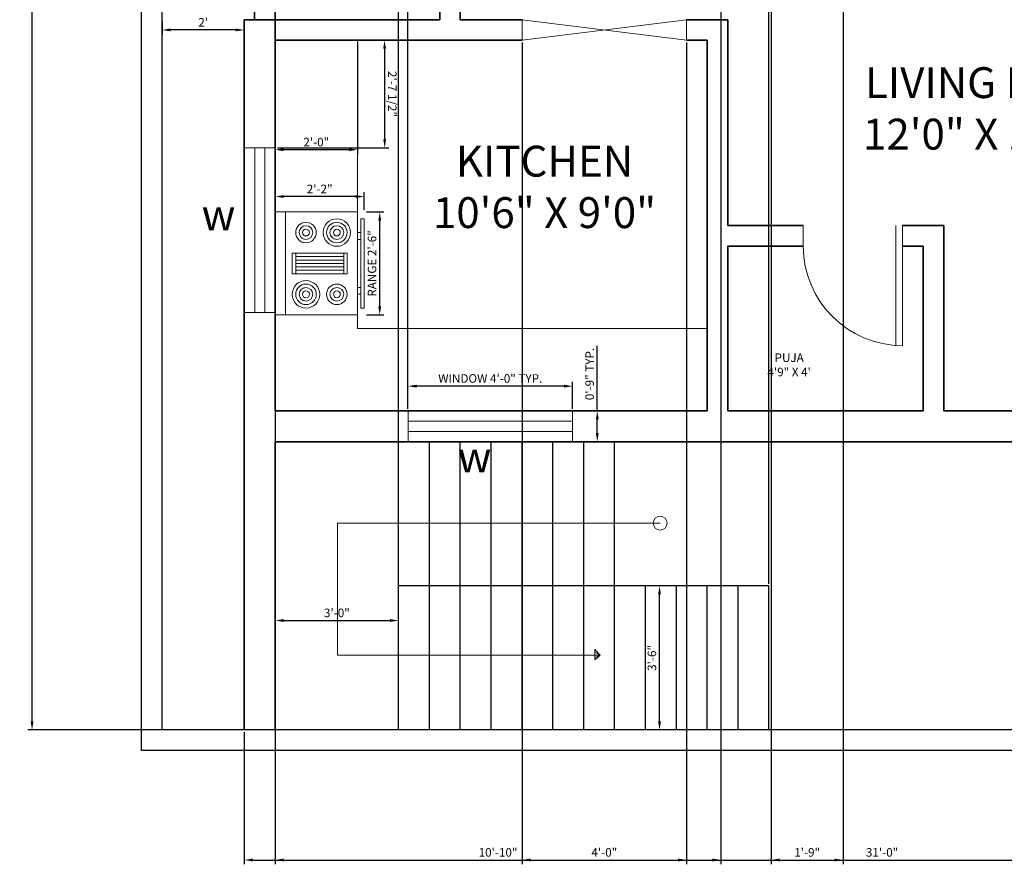
# Model space of a CAD drawing. Units: inches. Extents: x 1879 to 2382, y 1769 to 2461.
# Tile 1 of 5: x 1881 to 2168, y 1769 to 2015. Entities that reach past the tile are written whole.
import ezdxf

# ---------------------------------------------------------------- set-up
doc = ezdxf.new("R2010")
doc.units = ezdxf.units.IN
for name, color, linetype, lineweight in [('A-ANNO-DIMS', 2, 'Continuous', 18), ('A-ANNO-SYMB', 2, 'Continuous', 18), ('A-ANNO-TEXT', 3, 'Continuous', 18), ('A-AREA-IDEN', 7, 'Continuous', 18), ('A-DOOR', 3, 'Continuous', 18), ('A-EQPM', 8, 'Continuous', 18), ('A-FLOR-CASE', 8, 'Continuous', 18), ('A-FLOR-STRS', 7, 'Continuous', 25), ('A-GLAZ', 4, 'Continuous', 18), ('A-WALL', 7, 'Continuous', 35), ('C-PROP', 1, 'Continuous', 25)]:
    doc.layers.add(name, color=color, linetype=linetype, lineweight=lineweight)
doc.styles.get("Standard").update_dxf_attribs({"font": 'arial.ttf'})
doc.dimstyles.new('ISO-25', dxfattribs={"dimtxt": 2.5, "dimasz": 2.5, "dimexe": 1.25, "dimexo": 0.625, "dimtad": 1, "dimlunit": 4, "dimtxsty": 'Standard', "dimcen": 2.5, "dimadec": 0, "dimazin": 0, "dimtfac": 1, "dimtmove": 0, "dimatfit": 3, "dimfxl": 1, "dimarcsym": 0})

# ---------------------------------------------------------------- blocks, each defined once
blk = doc.blocks.new('Range-Oven - 30 in top')
for p, q in [((0, -3), (30, -3)), ((12, -6), (18, -6)), ((13, -20), (13, -6)), ((14, -6), (14, -20)), ((15, -20), (15, -6)), ((16, -6), (16, -20)), ((17, -20), (17, -6)), ((18, -20), (12, -20)), ((6, -24), (6, -25)), ((8, -25), (8, -24)), ((22, -25), (22, -24)), ((24, -24), (24, -25))]:
    blk.add_line(p, q)
for points in [[(0, -24), (0, 0), (30, 0), (30, -24)], [(12, -21), (12, -5), (18, -5), (18, -21)], [(2, -26), (2, -25), (28, -25), (28, -26)]]:
    blk.add_lwpolyline(points, close=True)
for centre, radius in [((6, -9), 4), ((6, -9), 3), ((6, -9), 2), ((6, -9), 1), ((24, -9), 3), ((24, -9), 2), ((24, -9), 1), ((24, -18), 4), ((6, -18), 3), ((6, -18), 2), ((6, -18), 1), ((24, -18), 3), ((24, -18), 2), ((24, -18), 1)]:
    blk.add_circle(centre, radius)
blk = doc.blocks.new('*D21')
at = {"layer": 'A-ANNO-DIMS', "color": 0, "lineweight": -2, "transparency": 16777216}
for p, q in [((1922.34, 2014.56), (1922.34, 2010.95)), ((1946.34, 2014.56), (1946.34, 2010.95)), ((1943.84, 2012.2), (1924.84, 2012.2))]:
    blk.add_line(p, q, dxfattribs=at)
at = {"layer": 'A-ANNO-DIMS', "color": 0, "transparency": 16777216}
for points in [[(1924.84, 2012.62), (1924.84, 2011.79), (1922.34, 2012.2)], [(1943.84, 2012.62), (1943.84, 2011.79), (1946.34, 2012.2)]]:
    blk.add_solid(points, dxfattribs=at)
at = {"layer": 'Defpoints', "color": 0, "transparency": 16777216}
for p in [(1922.34, 2015.18), (1946.34, 2015.18), (1922.34, 2012.2)]:
    blk.add_point(p, dxfattribs=at)
at = {"layer": 'A-ANNO-DIMS', "color": 0, "transparency": 16777216, "insert": (1934.34, 2014.08), "char_height": 2.5, "attachment_point": 5}
blk.add_mtext("2'", dxfattribs=at)
blk = doc.blocks.new('WN-48x9')
for p, q in [((0, 48), (0, 0)), ((9, 48), (0, 48)), ((3, 48), (3, 0)), ((6, 0), (6, 48)), ((9, 0), (9, 48)), ((0, 0), (9, 0))]:
    blk.add_line(p, q)
blk = doc.blocks.new('DR-SWING-29')
for p, q in [((27, 6), (27, 35)), ((29, 6), (29, 35)), ((0, 0), (0, 6)), ((27, 6), (27, 0)), ((29, 6), (29, 0))]:
    blk.add_line(p, q)
blk.add_arc((29, 6), 29, 90, 180)
blk = doc.blocks.new('*D29')
at = {"layer": 'A-ANNO-DIMS', "color": 0, "lineweight": -2, "transparency": 16777216}
for p, q in [((1994.08, 1901.81), (1994.08, 1909.63)), ((2042.08, 1901.81), (2042.08, 1909.63)), ((2039.58, 1908.38), (1996.58, 1908.38))]:
    blk.add_line(p, q, dxfattribs=at)
at = {"layer": 'A-ANNO-DIMS', "color": 0, "transparency": 16777216}
for points in [[(1996.58, 1908.8), (1996.58, 1907.96), (1994.08, 1908.38)], [(2039.58, 1908.8), (2039.58, 1907.96), (2042.08, 1908.38)]]:
    blk.add_solid(points, dxfattribs=at)
at = {"layer": 'Defpoints', "color": 0, "transparency": 16777216}
for p in [(1994.08, 1908.38), (1994.08, 1901.18), (2042.08, 1901.18)]:
    blk.add_point(p, dxfattribs=at)
at = {"layer": 'A-ANNO-DIMS', "color": 0, "transparency": 16777216, "insert": (2018.08, 1910.3), "char_height": 2.5, "attachment_point": 5}
blk.add_mtext('WINDOW 4\'-0" TYP.', dxfattribs=at)
blk = doc.blocks.new('*D30')
at = {"layer": 'A-ANNO-DIMS', "color": 0, "lineweight": -2, "transparency": 16777216}
for p, q in [((2049.28, 1901.18), (2049.28, 1920.17)), ((2042.71, 1901.18), (2050.53, 1901.18)), ((2049.28, 1894.68), (2049.28, 1898.68)), ((2042.71, 1892.18), (2050.53, 1892.18))]:
    blk.add_line(p, q, dxfattribs=at)
at = {"layer": 'A-ANNO-DIMS', "color": 0, "transparency": 16777216}
for points in [[(2048.87, 1898.68), (2049.7, 1898.68), (2049.28, 1901.18)], [(2048.87, 1894.68), (2049.7, 1894.68), (2049.28, 1892.18)]]:
    blk.add_solid(points, dxfattribs=at)
at = {"layer": 'Defpoints', "color": 0, "transparency": 16777216}
for p in [(2042.08, 1901.18), (2049.28, 1901.18), (2042.08, 1892.18)]:
    blk.add_point(p, dxfattribs=at)
at = {"layer": 'A-ANNO-DIMS', "color": 0, "transparency": 16777216, "insert": (2047.38, 1911.92), "char_height": 2.5, "attachment_point": 5, "rotation": 90}
blk.add_mtext('0\'-9" TYP.', dxfattribs=at)
blk = doc.blocks.new('*D53')
at = {"layer": 'A-ANNO-DIMS', "color": 0, "lineweight": -2, "transparency": 16777216}
for p, q in [((1981.96, 1959.14), (1987.08, 1959.14)), ((1985.83, 1931.64), (1985.83, 1956.64)), ((1981.96, 1929.14), (1987.08, 1929.14))]:
    blk.add_line(p, q, dxfattribs=at)
at = {"layer": 'A-ANNO-DIMS', "color": 0, "transparency": 16777216}
for points in [[(1985.41, 1956.64), (1986.25, 1956.64), (1985.83, 1959.14)], [(1985.41, 1931.64), (1986.25, 1931.64), (1985.83, 1929.14)]]:
    blk.add_solid(points, dxfattribs=at)
at = {"layer": 'Defpoints', "color": 0, "transparency": 16777216}
for p in [(1981.33, 1959.14), (1985.83, 1959.14), (1981.33, 1929.14)]:
    blk.add_point(p, dxfattribs=at)
at = {"layer": 'A-ANNO-DIMS', "color": 0, "transparency": 16777216, "insert": (1983.91, 1944.14), "char_height": 2.5, "attachment_point": 5, "rotation": 90}
blk.add_mtext('RANGE 2\'-6"', dxfattribs=at)
blk = doc.blocks.new('*D54')
at = {"layer": 'A-ANNO-DIMS', "color": 0, "lineweight": -2, "transparency": 16777216}
for p, q in [((1955.33, 1959.77), (1955.33, 1964.89)), ((1981.33, 1959.77), (1981.33, 1964.89)), ((1978.83, 1963.64), (1957.83, 1963.64))]:
    blk.add_line(p, q, dxfattribs=at)
at = {"layer": 'A-ANNO-DIMS', "color": 0, "transparency": 16777216}
for points in [[(1957.83, 1964.06), (1957.83, 1963.23), (1955.33, 1963.64)], [(1978.83, 1964.06), (1978.83, 1963.23), (1981.33, 1963.64)]]:
    blk.add_solid(points, dxfattribs=at)
at = {"layer": 'Defpoints', "color": 0, "transparency": 16777216}
for p in [(1955.33, 1963.64), (1955.33, 1959.14), (1981.33, 1959.14)]:
    blk.add_point(p, dxfattribs=at)
at = {"layer": 'A-ANNO-DIMS', "color": 0, "transparency": 16777216, "insert": (1968.33, 1965.52), "char_height": 2.5, "attachment_point": 5}
blk.add_mtext('2\'-2"', dxfattribs=at)
blk = doc.blocks.new('*D55')
at = {"layer": 'A-ANNO-DIMS', "color": 0, "lineweight": -2, "transparency": 16777216}
for p, q in [((1946.34, 1807.56), (1946.34, 1769.03)), ((2318.34, 1807.56), (2318.34, 1769.03)), ((1948.84, 1770.28), (2315.84, 1770.28))]:
    blk.add_line(p, q, dxfattribs=at)
at = {"layer": 'A-ANNO-DIMS', "color": 0, "transparency": 16777216}
for points in [[(1948.84, 1770.7), (1948.84, 1769.86), (1946.34, 1770.28)], [(2315.84, 1770.7), (2315.84, 1769.86), (2318.34, 1770.28)]]:
    blk.add_solid(points, dxfattribs=at)
at = {"layer": 'Defpoints', "color": 0, "transparency": 16777216}
for p in [(1946.34, 1808.18), (2318.34, 1808.18), (2318.34, 1770.28)]:
    blk.add_point(p, dxfattribs=at)
at = {"layer": 'A-ANNO-DIMS', "color": 0, "transparency": 16777216, "insert": (2132.34, 1772.18), "char_height": 2.5, "attachment_point": 5}
blk.add_mtext('31\'-0"', dxfattribs=at)
blk = doc.blocks.new('*D56')
at = {"layer": 'A-ANNO-DIMS', "color": 0, "lineweight": -2, "transparency": 16777216}
for p, q in [((1945.72, 2369.18), (1883.19, 2369.18)), ((1884.44, 1810.68), (1884.44, 2366.68)), ((1945.72, 1808.18), (1883.19, 1808.18))]:
    blk.add_line(p, q, dxfattribs=at)
at = {"layer": 'A-ANNO-DIMS', "color": 0, "transparency": 16777216}
for points in [[(1884.02, 2366.68), (1884.86, 2366.68), (1884.44, 2369.18)], [(1884.02, 1810.68), (1884.86, 1810.68), (1884.44, 1808.18)]]:
    blk.add_solid(points, dxfattribs=at)
at = {"layer": 'Defpoints', "color": 0, "transparency": 16777216}
for p in [(1884.44, 2369.18), (1946.34, 2369.18), (1946.34, 1808.18)]:
    blk.add_point(p, dxfattribs=at)
at = {"layer": 'A-ANNO-DIMS', "color": 0, "transparency": 16777216, "insert": (1882.54, 2088.68), "char_height": 2.5, "attachment_point": 5, "rotation": 90}
blk.add_mtext('46\'-9"', dxfattribs=at)
blk = doc.blocks.new('*D62')
at = {"layer": 'A-ANNO-DIMS', "color": 0, "lineweight": -2, "transparency": 16777216}
for p, q in [((2099.99, 2354.46), (2099.99, 1769.03)), ((2120.99, 2354.46), (2120.99, 1769.03)), ((2102.49, 1770.28), (2118.49, 1770.28))]:
    blk.add_line(p, q, dxfattribs=at)
at = {"layer": 'A-ANNO-DIMS', "color": 0, "transparency": 16777216}
for points in [[(2102.49, 1770.7), (2102.49, 1769.86), (2099.99, 1770.28)], [(2118.49, 1770.7), (2118.49, 1769.86), (2120.99, 1770.28)]]:
    blk.add_solid(points, dxfattribs=at)
at = {"layer": 'Defpoints', "color": 0, "transparency": 16777216}
for p in [(2099.99, 2355.08), (2120.99, 2355.08), (2120.99, 1770.28)]:
    blk.add_point(p, dxfattribs=at)
at = {"layer": 'A-ANNO-DIMS', "color": 0, "transparency": 16777216, "insert": (2110.49, 1772.18), "char_height": 2.5, "attachment_point": 5}
blk.add_mtext('1\'-9"', dxfattribs=at)
blk = doc.blocks.new('*D65')
at = {"layer": 'A-ANNO-DIMS', "color": 0, "lineweight": -2, "transparency": 16777216}
for p, q in [((1991.34, 1850.81), (1991.34, 2456.28)), ((2099.34, 1850.81), (2099.34, 2456.28)), ((1993.84, 2455.03), (2096.84, 2455.03))]:
    blk.add_line(p, q, dxfattribs=at)
at = {"layer": 'A-ANNO-DIMS', "color": 0, "transparency": 16777216}
for points in [[(1993.84, 2455.44), (1993.84, 2454.61), (1991.34, 2455.03)], [(2096.84, 2455.44), (2096.84, 2454.61), (2099.34, 2455.03)]]:
    blk.add_solid(points, dxfattribs=at)
at = {"layer": 'Defpoints', "color": 0, "transparency": 16777216}
for p in [(2099.34, 2455.03), (1991.34, 1850.18), (2099.34, 1850.18)]:
    blk.add_point(p, dxfattribs=at)
at = {"layer": 'A-ANNO-DIMS', "color": 0, "transparency": 16777216, "insert": (2045.34, 2456.93), "char_height": 2.5, "attachment_point": 5}
blk.add_mtext('9\'-0"', dxfattribs=at)
blk = doc.blocks.new('*D66')
at = {"layer": 'A-ANNO-DIMS', "color": 0, "lineweight": -2, "transparency": 16777216}
for p, q in [((2098.72, 1850.18), (2066.19, 1850.18)), ((2067.44, 1810.68), (2067.44, 1847.68)), ((2098.72, 1808.18), (2066.19, 1808.18))]:
    blk.add_line(p, q, dxfattribs=at)
at = {"layer": 'A-ANNO-DIMS', "color": 0, "transparency": 16777216}
for points in [[(2067.02, 1847.68), (2067.86, 1847.68), (2067.44, 1850.18)], [(2067.02, 1810.68), (2067.86, 1810.68), (2067.44, 1808.18)]]:
    blk.add_solid(points, dxfattribs=at)
at = {"layer": 'Defpoints', "color": 0, "transparency": 16777216}
for p in [(2067.44, 1850.18), (2099.34, 1850.18), (2099.34, 1808.18)]:
    blk.add_point(p, dxfattribs=at)
at = {"layer": 'A-ANNO-DIMS', "color": 0, "transparency": 16777216, "insert": (2065.54, 1829.18), "char_height": 2.5, "attachment_point": 5, "rotation": 90}
blk.add_mtext('3\'-6"', dxfattribs=at)
blk = doc.blocks.new('*D67')
at = {"layer": 'A-ANNO-DIMS', "color": 0, "lineweight": -2, "transparency": 16777216}
for p, q in [((1955.34, 1901.81), (1955.34, 2456.28)), ((1994.08, 1901.81), (1994.08, 2456.28)), ((1957.84, 2455.03), (1991.58, 2455.03))]:
    blk.add_line(p, q, dxfattribs=at)
at = {"layer": 'A-ANNO-DIMS', "color": 0, "transparency": 16777216}
for points in [[(1957.84, 2455.44), (1957.84, 2454.61), (1955.34, 2455.03)], [(1991.58, 2455.44), (1991.58, 2454.61), (1994.08, 2455.03)]]:
    blk.add_solid(points, dxfattribs=at)
at = {"layer": 'Defpoints', "color": 0, "transparency": 16777216}
for p in [(1994.08, 2455.03), (1955.34, 1901.18), (1994.08, 1901.18)]:
    blk.add_point(p, dxfattribs=at)
at = {"layer": 'A-ANNO-DIMS', "color": 0, "transparency": 16777216, "insert": (1974.71, 2456.95), "char_height": 2.5, "attachment_point": 5}
blk.add_mtext('3\'-2 1/2"', dxfattribs=at)
blk = doc.blocks.new('*D68')
at = {"layer": 'A-ANNO-DIMS', "color": 0, "lineweight": -2, "transparency": 16777216}
for p, q in [((1955.34, 2008.56), (1955.34, 1976.03)), ((1979.34, 2008.56), (1979.34, 1976.03)), ((1976.84, 1977.28), (1957.84, 1977.28))]:
    blk.add_line(p, q, dxfattribs=at)
at = {"layer": 'A-ANNO-DIMS', "color": 0, "transparency": 16777216}
for points in [[(1957.84, 1977.7), (1957.84, 1976.86), (1955.34, 1977.28)], [(1976.84, 1977.7), (1976.84, 1976.86), (1979.34, 1977.28)]]:
    blk.add_solid(points, dxfattribs=at)
at = {"layer": 'Defpoints', "color": 0, "transparency": 16777216}
for p in [(1955.34, 2009.18), (1979.34, 2009.18), (1955.34, 1977.28)]:
    blk.add_point(p, dxfattribs=at)
at = {"layer": 'A-ANNO-DIMS', "color": 0, "transparency": 16777216, "insert": (1967.34, 1979.18), "char_height": 2.5, "attachment_point": 5}
blk.add_mtext('2\'-0"', dxfattribs=at)
blk = doc.blocks.new('*D70')
at = {"layer": 'A-ANNO-DIMS', "color": 0, "lineweight": -2, "transparency": 16777216}
for p, q in [((2027.34, 2008.56), (2027.34, 1769.03)), ((2075.34, 2008.56), (2075.34, 1769.03)), ((2029.84, 1770.28), (2072.84, 1770.28))]:
    blk.add_line(p, q, dxfattribs=at)
at = {"layer": 'A-ANNO-DIMS', "color": 0, "transparency": 16777216}
for points in [[(2029.84, 1770.7), (2029.84, 1769.86), (2027.34, 1770.28)], [(2072.84, 1770.7), (2072.84, 1769.86), (2075.34, 1770.28)]]:
    blk.add_solid(points, dxfattribs=at)
at = {"layer": 'Defpoints', "color": 0, "transparency": 16777216}
for p in [(2027.34, 2009.18), (2075.34, 2009.18), (2075.34, 1770.28)]:
    blk.add_point(p, dxfattribs=at)
at = {"layer": 'A-ANNO-DIMS', "color": 0, "transparency": 16777216, "insert": (2051.34, 1772.18), "char_height": 2.5, "attachment_point": 5}
blk.add_mtext('4\'-0"', dxfattribs=at)
blk = doc.blocks.new('*D71')
at = {"layer": 'A-ANNO-DIMS', "color": 0, "lineweight": -2, "transparency": 16777216}
for p, q in [((1955.34, 2362.56), (1955.34, 1769.03)), ((2085.34, 2362.56), (2085.34, 1769.03)), ((1957.84, 1770.28), (2082.84, 1770.28))]:
    blk.add_line(p, q, dxfattribs=at)
at = {"layer": 'A-ANNO-DIMS', "color": 0, "transparency": 16777216}
for points in [[(1957.84, 1770.7), (1957.84, 1769.86), (1955.34, 1770.28)], [(2082.84, 1770.7), (2082.84, 1769.86), (2085.34, 1770.28)]]:
    blk.add_solid(points, dxfattribs=at)
at = {"layer": 'Defpoints', "color": 0, "transparency": 16777216}
for p in [(1955.34, 2363.18), (2085.34, 2363.18), (2085.34, 1770.28)]:
    blk.add_point(p, dxfattribs=at)
at = {"layer": 'A-ANNO-DIMS', "color": 0, "transparency": 16777216, "insert": (2020.34, 1772.18), "char_height": 2.5, "attachment_point": 5}
blk.add_mtext('10\'-10"', dxfattribs=at)
blk = doc.blocks.new('*D75')
at = {"layer": 'A-ANNO-DIMS', "color": 0, "lineweight": -2, "transparency": 16777216}
for p, q in [((1955.97, 2009.18), (1988.49, 2009.22)), ((1987.24, 2006.72), (1987.27, 1980.34)), ((1956, 1977.81), (1988.53, 1977.84))]:
    blk.add_line(p, q, dxfattribs=at)
at = {"layer": 'A-ANNO-DIMS', "color": 0, "transparency": 16777216}
for points in [[(1987.66, 2006.72), (1986.83, 2006.71), (1987.24, 2009.22)], [(1987.69, 1980.34), (1986.86, 1980.34), (1987.28, 1977.84)]]:
    blk.add_solid(points, dxfattribs=at)
at = {"layer": 'Defpoints', "color": 0, "transparency": 16777216}
for p in [(1955.34, 2009.18), (1955.38, 1977.81), (1987.28, 1977.84)]:
    blk.add_point(p, dxfattribs=at)
at = {"layer": 'A-ANNO-DIMS', "color": 0, "transparency": 16777216, "insert": (1989.18, 1993.53), "char_height": 2.5, "attachment_point": 5, "rotation": 270.0621}
blk.add_mtext('2\'-7 1/2"', dxfattribs=at)
blk = doc.blocks.new('*D77')
at = {"layer": 'A-ANNO-DIMS', "color": 0, "lineweight": -2, "transparency": 16777216}
for p, q in [((1955.34, 1808.81), (1955.34, 1841.33)), ((1991.34, 1808.81), (1991.34, 1841.33)), ((1957.84, 1840.08), (1988.84, 1840.08))]:
    blk.add_line(p, q, dxfattribs=at)
at = {"layer": 'A-ANNO-DIMS', "color": 0, "transparency": 16777216}
for points in [[(1957.84, 1840.5), (1957.84, 1839.66), (1955.34, 1840.08)], [(1988.84, 1840.5), (1988.84, 1839.66), (1991.34, 1840.08)]]:
    blk.add_solid(points, dxfattribs=at)
at = {"layer": 'Defpoints', "color": 0, "transparency": 16777216}
for p in [(1991.34, 1840.08), (1955.34, 1808.18), (1991.34, 1808.18)]:
    blk.add_point(p, dxfattribs=at)
at = {"layer": 'A-ANNO-DIMS', "color": 0, "transparency": 16777216, "insert": (1973.34, 1841.98), "char_height": 2.5, "attachment_point": 5}
blk.add_mtext('3\'-0"', dxfattribs=at)

msp = doc.modelspace()

# ---------------------------------------------------------------- linework, layer by layer
at = {"layer": 'A-ANNO-SYMB'}
for p, q in [((2067.6, 1868.438), (1973.565, 1868.438)), ((1973.565, 1868.438), (1973.565, 1830)), ((1973.565, 1830), (2048.579, 1830)), ((2048.579, 1828.656), (2048.579, 1831.672)), ((2048.579, 1831.672), (2048.579, 1830.072)), ((2048.579, 1830.072), (2048.579, 1831.672)), ((2048.579, 1831.672), (2048.579, 1829.99)), ((2048.579, 1831.672), (2050.076, 1829.969)), ((2050.076, 1829.969), (2048.579, 1830.831)), ((2048.579, 1830.831), (2050.076, 1829.969)), ((2048.579, 1828.656), (2048.579, 1830.031)), ((2048.579, 1830), (2048.579, 1828.656)), ((2048.579, 1829.99), (2048.579, 1828.656)), ((2050.076, 1829.969), (2048.579, 1828.656)), ((2048.579, 1828.656), (2048.579, 1829.969)), ((2048.579, 1829.969), (2050.076, 1829.969)), ((2050.076, 1829.969), (2048.579, 1829.344))]:
    msp.add_line(p, q, dxfattribs=at)
msp.add_circle((2067.6, 1868.438), 2.029, dxfattribs=at)
at = {"layer": 'A-DOOR'}
for p, q in [((2027.341, 2015.18), (2027.341, 2009.18)), ((2075.341, 2009.18), (2027.341, 2015.18)), ((2027.341, 2015.18), (2027.341, 2009.18)), ((2027.341, 2009.18), (2075.341, 2015.18)), ((2075.341, 2009.18), (2075.341, 2015.18))]:
    msp.add_line(p, q, dxfattribs=at)
at = {"layer": 'A-FLOR-CASE'}
for p, q in [((1979.341, 1925.18), (1979.341, 2009.18)), ((2081.341, 1925.18), (1979.341, 1925.18))]:
    msp.add_line(p, q, dxfattribs=at)
at = {"layer": 'A-FLOR-STRS'}
for p, q in [((1991.341, 1808.18), (1991.341, 1892.18)), ((2000.341, 1808.18), (2000.341, 1892.18)), ((2009.341, 1808.18), (2009.341, 1892.18)), ((2018.341, 1808.18), (2018.341, 1892.18)), ((2027.341, 1808.18), (2027.341, 1892.18)), ((2036.341, 1808.18), (2036.341, 1892.18)), ((2045.341, 1808.18), (2045.341, 1892.18)), ((2054.341, 1808.18), (2054.341, 1892.18)), ((2099.341, 1850.18), (1991.341, 1850.18)), ((2063.341, 1808.18), (2063.341, 1850.18)), ((2072.341, 1808.18), (2072.341, 1850.18)), ((2081.341, 1808.18), (2081.341, 1850.18)), ((2090.341, 1808.18), (2090.341, 1850.18)), ((2099.341, 1808.18), (2099.341, 1850.18))]:
    msp.add_line(p, q, dxfattribs=at)
at = {"layer": 'A-WALL'}
for p, q in [((1949.341, 2015.18), (1949.341, 2135.18)), ((1955.341, 2015.18), (1955.341, 2135.18)), ((2003.341, 2015.18), (2003.341, 2135.18)), ((2009.341, 2015.18), (2009.341, 2135.18)), ((1946.341, 1808.18), (1946.341, 2015.18)), ((1955.341, 2015.18), (1946.341, 2015.18)), ((2003.341, 2015.18), (1955.341, 2015.18)), ((2027.341, 2015.18), (2009.341, 2015.18)), ((2087.341, 2015.18), (2075.341, 2015.18)), ((2087.341, 1955.18), (2087.341, 2015.18)), ((1955.341, 1901.18), (1955.341, 2009.18)), ((2027.341, 2009.18), (1955.341, 2009.18)), ((2081.341, 2009.18), (2075.341, 2009.18)), ((2081.341, 2009.18), (2075.341, 2009.18)), ((2081.341, 1901.18), (2081.341, 2009.18)), ((2109.341, 1955.18), (2087.341, 1955.18)), ((2150.341, 1955.18), (2138.341, 1955.18)), ((2150.341, 1901.18), (2150.341, 1955.18)), ((2087.341, 1901.18), (2087.341, 1949.18)), ((2109.341, 1949.18), (2087.341, 1949.18)), ((2144.341, 1949.18), (2138.341, 1949.18)), ((2144.341, 1949.18), (2138.341, 1949.18)), ((2144.341, 1901.18), (2144.341, 1949.18)), ((2081.341, 1901.18), (1955.341, 1901.18)), ((2144.341, 1901.18), (2087.341, 1901.18)), ((2237.341, 1901.18), (2150.341, 1901.18)), ((1955.341, 1808.18), (1955.341, 1892.18)), ((2237.341, 1892.18), (1955.341, 1892.18))]:
    msp.add_line(p, q, dxfattribs=at)
at = {"layer": 'C-PROP'}
for p, q in [((1916.341, 1802.18), (1916.341, 2402.18)), ((1922.341, 1808.18), (1922.341, 2396.18)), ((2342.341, 1808.18), (1922.341, 1808.18)), ((2348.341, 1802.18), (1916.341, 1802.18))]:
    msp.add_line(p, q, dxfattribs=at)

# ---------------------------------------------------------------- block references
at = {"layer": 'A-DOOR', "extrusion": (0, 0, -1), "zscale": -1, "rotation": 180}
msp.add_blockref('DR-SWING-29', (-2109.341, 1955.18), dxfattribs=at)
at = {"layer": 'A-EQPM', "rotation": 90}
msp.add_blockref('Range-Oven - 30 in top', (1955.331, 1929.144), dxfattribs=at)
at = {"layer": 'A-GLAZ'}
for p, rotation in [((1955.375, 1977.805), 180), ((2042.083, 1892.18), 89.99999999999896)]:
    msp.add_blockref('WN-48x9', p, dxfattribs=dict(at, rotation=rotation))

# ---------------------------------------------------------------- texts
at = {"layer": 'A-ANNO-TEXT', "char_height": 9, "attachment_point": 1}
for insert in [(1882.7, 1962.828), (1957.363, 1892.245)]:
    msp.add_mtext_dynamic_manual_height_columns('\\pxqc;w', width=112.22887, gutter_width=12.5, heights=[0], dxfattribs=dict(at, insert=insert))
at = {"layer": 'A-AREA-IDEN', "attachment_point": 1}
for s, width, insert, char_height in [('\\pxqc;LIVING HALL\\P12\'0" X 18\'6"', 86.0711, (2119.688, 2001.337), 9), ('\\pxqc;KITCHEN\\P10\'6" X 9\'0"', 65.64687, (2001.069, 1978.454), 9), ('\\pxqc;PUJA\\P4\'9" X 4\'', 41.02934, (2084.725, 1917.93), 2.5)]:
    msp.add_mtext_dynamic_manual_height_columns(s, width=width, gutter_width=12.5, heights=[0], dxfattribs=dict(at, insert=insert, char_height=char_height))

# ---------------------------------------------------------------- dimensions: what is measured, and where the dimension line sits
at = {"layer": 'A-ANNO-DIMS'}
for base, p1, p2, override, picture, middle in [((1994.083, 2455.028), (1955.341, 1901.18), (1994.083, 1901.18), {"dimdec": 1, "dimlfac": 1, "dimrnd": 0, "dimzin": 1, "dimdsep": 46, "dimlunit": 4, "dimfrac": 2}, '*D67', (1974.712, 2456.946)), ((2099.341, 2455.028), (1991.341, 1850.18), (2099.341, 1850.18), {"dimdec": 1, "dimlfac": 1, "dimrnd": 0, "dimzin": 1, "dimdsep": 46, "dimlunit": 4, "dimfrac": 2}, '*D65', (2045.341, 2456.929)), ((2085.341, 1770.28), (1955.341, 2363.18), (2085.341, 2363.18), {"dimdec": 1, "dimlfac": 1, "dimrnd": 0, "dimzin": 1, "dimdsep": 46, "dimlunit": 4, "dimfrac": 2}, '*D71', (2020.341, 1772.182)), ((2120.987, 1770.28), (2099.987, 2355.082), (2120.987, 2355.082), {"dimdec": 1, "dimlfac": 1, "dimrnd": 0, "dimzin": 1, "dimdsep": 46, "dimlunit": 4, "dimfrac": 2}, '*D62', (2110.487, 1772.182)), ((1922.341, 2012.202), (1946.341, 2015.18), (1922.341, 2015.18), {"dimclrd": 0, "dimclre": 0, "dimclrt": 0}, '*D21', (1934.341, 2014.082)), ((2075.341, 1770.28), (2027.341, 2009.18), (2075.341, 2009.18), {"dimdec": 1, "dimlfac": 1, "dimrnd": 0, "dimzin": 1, "dimdsep": 46, "dimlunit": 4, "dimfrac": 2}, '*D70', (2051.341, 1772.182)), ((1991.341, 1840.08), (1955.341, 1808.18), (1991.341, 1808.18), {"dimdec": 1, "dimlfac": 1, "dimrnd": 0, "dimzin": 1, "dimdsep": 46, "dimlunit": 4, "dimfrac": 2}, '*D77', (1973.341, 1841.983)), ((2318.341, 1770.28), (1946.341, 1808.18), (2318.341, 1808.18), {"dimdec": 1, "dimlfac": 1, "dimrnd": 0, "dimzin": 1, "dimdsep": 46, "dimlunit": 4, "dimfrac": 2}, '*D55', (2132.341, 1772.183))]:
    dim = msp.add_linear_dim(base=base, p1=p1, p2=p2, dimstyle='ISO-25', override=override, dxfattribs=at)
    dim.commit()
    dim.dimension.update_dxf_attribs({"geometry": picture, "text_midpoint": middle})
for base, p1, p2, angle, picture, middle in [((1884.441, 2369.18), (1946.341, 1808.18), (1946.341, 2369.18), 90, '*D56', (1882.54, 2088.68)), ((1987.275, 1977.84), (1955.341, 2009.18), (1955.375, 1977.805), 270.06207, '*D75', (1989.176, 1993.529)), ((1955.341, 1977.28), (1979.341, 2009.18), (1955.341, 2009.18), 180, '*D68', (1967.341, 1979.182)), ((1955.331, 1963.644), (1981.331, 1959.144), (1955.331, 1959.144), 180, '*D54', (1968.331, 1965.524)), ((2067.441, 1850.18), (2099.341, 1808.18), (2099.341, 1850.18), 90, '*D66', (2065.539, 1829.18))]:
    dim = msp.add_linear_dim(base=base, p1=p1, p2=p2, angle=angle, dimstyle='ISO-25', override={"dimdec": 1, "dimlfac": 1, "dimrnd": 0, "dimzin": 1, "dimdsep": 46, "dimlunit": 4, "dimfrac": 2}, dxfattribs=at)
    dim.commit()
    dim.dimension.update_dxf_attribs({"geometry": picture, "text_midpoint": middle})
for base, p1, p2, angle, text, picture, middle in [((1985.831, 1959.144), (1981.331, 1929.144), (1981.331, 1959.144), 90, 'RANGE <>', '*D53', (1983.913, 1944.144)), ((2049.283, 1901.18), (2042.083, 1892.18), (2042.083, 1901.18), 90, '<> TYP.', '*D30', (2047.382, 1911.925)), ((1994.083, 1908.38), (2042.083, 1901.18), (1994.083, 1901.18), 180, 'WINDOW <> TYP.', '*D29', (2018.083, 1910.299))]:
    dim = msp.add_linear_dim(base=base, p1=p1, p2=p2, angle=angle, text=text, dimstyle='ISO-25', override={"dimdec": 1, "dimlfac": 1, "dimrnd": 0, "dimzin": 1, "dimdsep": 46, "dimlunit": 4, "dimfrac": 2}, dxfattribs=at)
    dim.commit()
    dim.dimension.update_dxf_attribs({"geometry": picture, "text_midpoint": middle})

doc.saveas('drawing.dxf')
